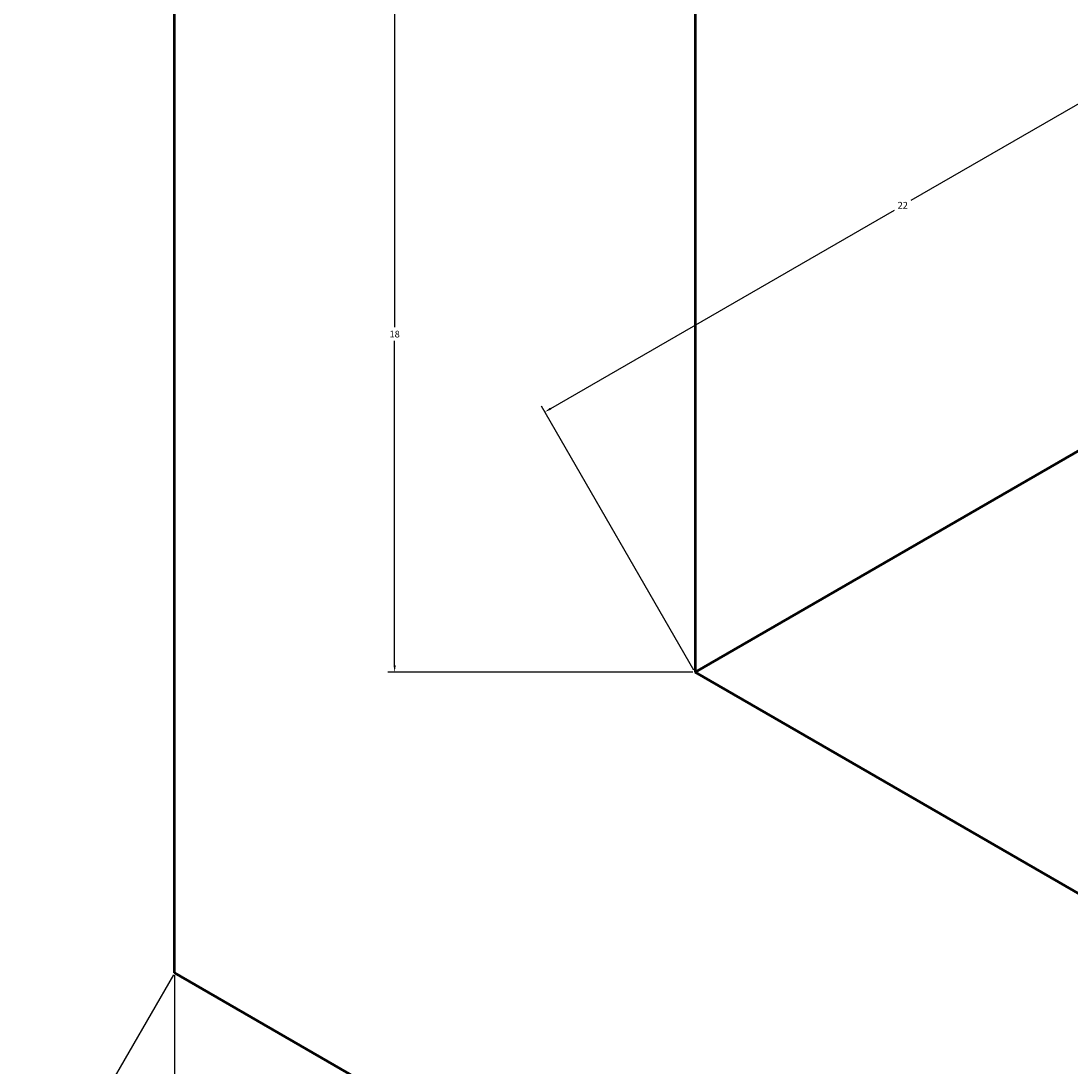
# Model space of a CAD drawing. Units: millimetres. Extents: x 2919 to 3075, y 2801 to 2951.
# Tile 2 of 14: x 2924 to 2952, y 2854 to 2882. Entities that reach past the tile are written whole.
import ezdxf

# ---------------------------------------------------------------- set-up
doc = ezdxf.new("R2010")
doc.units = ezdxf.units.MM
doc.layers.add('M-DIMS', color=2, linetype='Continuous', lineweight=18)
doc.layers.add('M-OUTL', color=7, linetype='Continuous', lineweight=50)
doc.styles.get("Standard").update_dxf_attribs({"font": 'arial.ttf'})
doc.dimstyles.get("Standard").update_dxf_attribs({"dimtxt": 0.18, "dimasz": 0.18, "dimexe": 0.18, "dimexo": 0.0625, "dimgap": 0.09, "dimtad": 0, "dimtih": 1, "dimtoh": 1, "dimdec": 4, "dimzin": 0, "dimdsep": 46, "dimtxsty": 'Standard', "dimcen": 0.09, "dimadec": 0, "dimazin": 0, "dimtfac": 1, "dimtdec": 4, "dimtofl": 0, "dimtmove": 0, "dimatfit": 3, "dimfxl": 1, "dimtolj": 1, "dimtzin": 0, "dimarcsym": 0})

# ---------------------------------------------------------------- blocks, each defined once
blk = doc.blocks.new('*D2')
at = {"layer": 'Defpoints', "color": 0, "transparency": 16777216}
for p in [(2927.773, 2856.893), (3066.337, 2840.893), (3066.337, 2800.893)]:
    blk.add_point(p, dxfattribs=at)
at = {"layer": 'M-DIMS', "color": 0, "lineweight": -2, "transparency": 16777216}
for p, q in [((2927.773, 2856.831), (2927.773, 2800.713)), ((3066.337, 2840.831), (3066.337, 2800.713)), ((2927.953, 2800.893), (2996.6, 2800.893)), ((3066.157, 2800.893), (2997.51, 2800.893))]:
    blk.add_line(p, q, dxfattribs=at)
at = {"layer": 'M-DIMS', "color": 0, "transparency": 16777216}
for points in [[(2927.953, 2800.923), (2927.953, 2800.863), (2927.773, 2800.893)], [(3066.157, 2800.923), (3066.157, 2800.863), (3066.337, 2800.893)]]:
    blk.add_solid(points, dxfattribs=at)
at = {"layer": 'M-DIMS', "color": 0, "transparency": 16777216, "insert": (2997.055, 2800.893), "char_height": 0.18, "attachment_point": 5}
blk.add_mtext('\\A1;138.56', dxfattribs=at)
blk = doc.blocks.new('*D3')
at = {"layer": 'Defpoints', "color": 0, "transparency": 16777216}
for p in [(2927.773, 2856.893), (2923.773, 2849.965), (3010.912, 2808.893)]:
    blk.add_point(p, dxfattribs=at)
at = {"layer": 'M-DIMS', "color": 0, "lineweight": -2, "transparency": 16777216}
for p, q in [((2927.742, 2856.839), (2923.683, 2849.809)), ((2923.929, 2849.875), (2965.124, 2826.091)), ((3006.756, 2802.055), (2965.561, 2825.839)), ((3010.88, 2808.839), (3006.822, 2801.809))]:
    blk.add_line(p, q, dxfattribs=at)
at = {"layer": 'M-DIMS', "color": 0, "transparency": 16777216}
for points in [[(2923.944, 2849.901), (2923.914, 2849.849), (2923.773, 2849.965)], [(3006.771, 2802.081), (3006.741, 2802.029), (3006.912, 2801.965)]]:
    blk.add_solid(points, dxfattribs=at)
at = {"layer": 'M-DIMS', "color": 0, "transparency": 16777216, "insert": (2965.342, 2825.965), "char_height": 0.18, "attachment_point": 5}
blk.add_mtext('\\A1;96', dxfattribs=at)
blk = doc.blocks.new('*D10')
at = {"layer": 'Defpoints', "color": 0, "transparency": 16777216}
for p in [(2956.682, 2882.821), (2960.682, 2875.893), (2941.63, 2864.893)]:
    blk.add_point(p, dxfattribs=at)
at = {"layer": 'M-DIMS', "color": 0, "lineweight": -2, "transparency": 16777216}
for p, q in [((2956.526, 2882.731), (2947.375, 2877.448)), ((2960.651, 2875.947), (2956.592, 2882.977)), ((2937.785, 2871.911), (2946.936, 2877.195)), ((2941.598, 2864.947), (2937.54, 2871.977))]:
    blk.add_line(p, q, dxfattribs=at)
at = {"layer": 'M-DIMS', "color": 0, "transparency": 16777216}
for points in [[(2956.511, 2882.757), (2956.541, 2882.705), (2956.682, 2882.821)], [(2937.77, 2871.937), (2937.8, 2871.885), (2937.63, 2871.821)]]:
    blk.add_solid(points, dxfattribs=at)
at = {"layer": 'M-DIMS', "color": 0, "transparency": 16777216, "insert": (2947.156, 2877.321), "char_height": 0.18, "attachment_point": 5}
blk.add_mtext('\\A1;22', dxfattribs=at)
blk = doc.blocks.new('*D15')
at = {"layer": 'Defpoints', "color": 0, "transparency": 16777216}
for p in [(2933.63, 2882.893), (2941.63, 2882.893), (2941.63, 2864.893)]:
    blk.add_point(p, dxfattribs=at)
at = {"layer": 'M-DIMS', "color": 0, "lineweight": -2, "transparency": 16777216}
for p, q in [((2941.567, 2882.893), (2933.45, 2882.893)), ((2933.63, 2882.713), (2933.63, 2874.075)), ((2933.63, 2865.073), (2933.63, 2873.711)), ((2941.567, 2864.893), (2933.45, 2864.893))]:
    blk.add_line(p, q, dxfattribs=at)
at = {"layer": 'M-DIMS', "color": 0, "transparency": 16777216}
for points in [[(2933.6, 2882.713), (2933.66, 2882.713), (2933.63, 2882.893)], [(2933.6, 2865.073), (2933.66, 2865.073), (2933.63, 2864.893)]]:
    blk.add_solid(points, dxfattribs=at)
at = {"layer": 'M-DIMS', "color": 0, "transparency": 16777216, "insert": (2933.63, 2873.893), "char_height": 0.18, "attachment_point": 5}
blk.add_mtext('\\A1;18', dxfattribs=at)

msp = doc.modelspace()

# ---------------------------------------------------------------- linework, layer by layer
at = {"layer": 'M-OUTL'}
for p, q in [((2927.7732, 2856.8932), (2927.7732, 2890.8932)), ((2941.6296, 2882.8932), (2941.6296, 2864.8932)), ((2941.6296, 2864.8932), (2960.6821, 2875.8932)), ((2941.6296, 2864.8932), (2960.6821, 2875.8932)), ((2941.6296, 2864.8932), (2960.6821, 2875.8932)), ((3010.9116, 2824.8932), (2941.6296, 2864.8932)), ((2927.7732, 2856.8932), (3010.9116, 2808.8932))]:
    msp.add_line(p, q, dxfattribs=at)

# ---------------------------------------------------------------- dimensions: what is measured, and where the dimension line sits
at = {"layer": 'M-DIMS'}
for base, p1, p2, angle, picture, middle in [((2933.6296, 2882.8932), (2941.6296, 2864.8932), (2941.6296, 2882.8932), 90, '*D15', (2933.6296, 2873.8932)), ((2956.6821, 2882.8214), (2941.6296, 2864.8932), (2960.6821, 2875.8932), 30, '*D10', (2947.1559, 2877.3214)), ((2923.7732, 2849.965), (3010.9116, 2808.8932), (2927.7732, 2856.8932), 150, '*D3', (2965.3424, 2825.965))]:
    dim = msp.add_linear_dim(base=base, p1=p1, p2=p2, angle=angle, dimstyle='Standard', override={"dimdec": 0, "dimlfac": 1, "dimrnd": 0, "dimzin": 0, "dimdsep": 46, "dimlunit": 2}, dxfattribs=at)
    dim.commit()
    dim.dimension.update_dxf_attribs({"geometry": picture, "text_midpoint": middle})
dim = msp.add_linear_dim(base=(3066.3372, 2800.8932), p1=(2927.7732, 2856.8932), p2=(3066.3372, 2840.8932), dimstyle='Standard', override={"dimdec": 2, "dimlfac": 1, "dimrnd": 0, "dimzin": 0, "dimdsep": 46, "dimlunit": 2}, dxfattribs=at)
dim.commit()
dim.dimension.update_dxf_attribs({"geometry": '*D2', "text_midpoint": (2997.0552, 2800.8932)})

doc.saveas('drawing.dxf')
